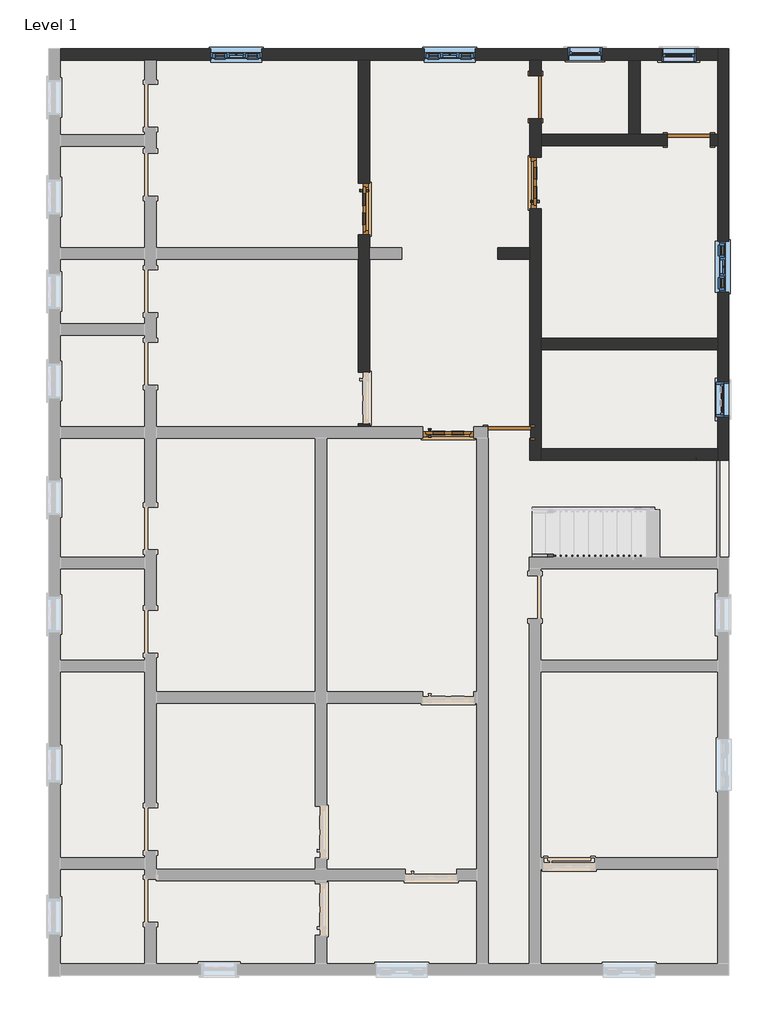
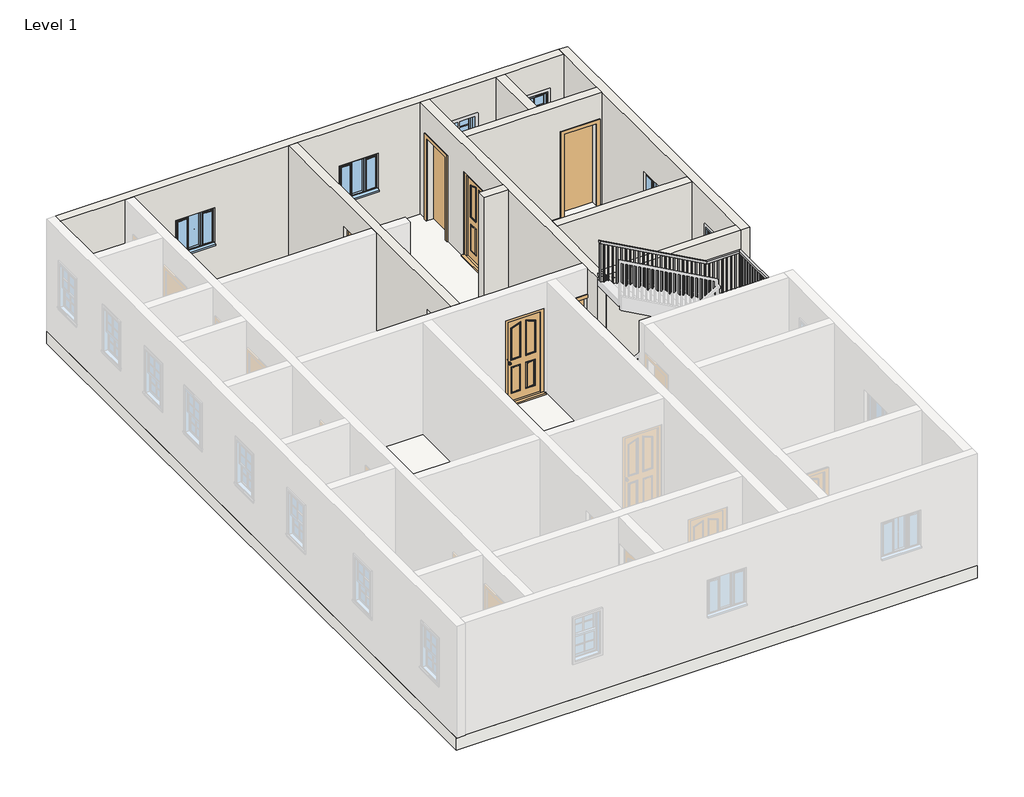
# One storey, part 2 of 3: 9 walls, 6 doors, 6 windows, 1 railing, 1 slab.
# Revit data of these elements (continued)
# Element 22 (IfcWindow, "Windows_Tpl_w-Glazing_Cross-Bars : 910x910mm") (continued)
#   Materials on its faces: "Window Frame", "Glass"
# Element 23 (IfcWindow, "Windows_Tpl_w-Glazing_Cross-Bars : 910x910mm")
#   Mark = "17"
#   Phase Created = New Construction
#   Materials on its faces: "Window Frame", "Glass"
# Materials
#   "Door - Glazing": colour RGB 0 0 255, transparency 0.75
#   "Door - Panel": class "Wood", colour RGB 210 159 95, transparency 0, Cost = 0
#   "Door - Frame/Mullion": class "Wood", colour RGB 212 179 113, transparency 0
#   "Door - Handle": colour RGB 246 240 166, transparency 0
#   "Door - Frame": colour RGB 118 70 51, transparency 0, Cost = 0
#   "Wood - Stained": class "Wood", colour RGB 224 178 126, transparency 0, Cost = 0
#   "Clad - White": class "Wood", colour RGB 242 242 238, transparency 0, Cost = 0
#   "Glass": class "Glass", colour RGB 0 128 192, transparency 0.75, Description = "Soda Lime Glass", Cost = 0
#   "Window Frame": colour RGB 249 249 249, transparency 0
#   "Default Floor": colour RGB 128 128 128, transparency 0, Cost = 0
#   "Default Wall": colour RGB 128 128 128, transparency 0, Cost = 0
#   "Tile, Porcelain, 4in": class "Generic", colour RGB 89 87 158, transparency 0, Description = "Porcelain tile, 4\", white", Cost = 0
